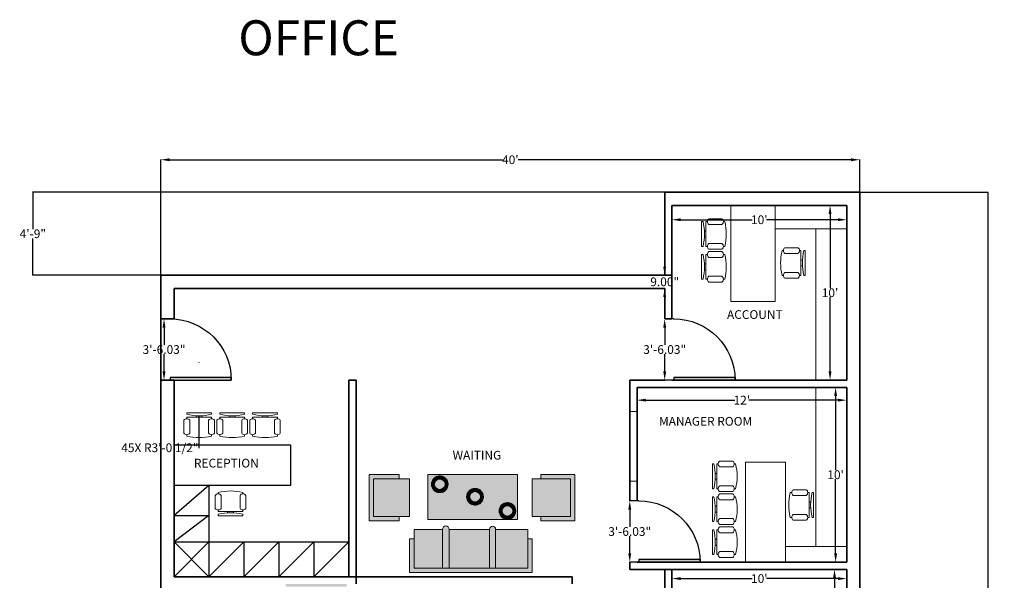
# Model space of a CAD drawing. Units: inches. Extents: x -57 to 1512, y -896 to 149.
# Tile 6 of 6: x 835 to 1512, y -261 to 124. Entities that reach past the tile are written whole.
import ezdxf

# ---------------------------------------------------------------- set-up
doc = ezdxf.new("R2010")
doc.units = ezdxf.units.IN
doc.header["$MEASUREMENT"] = 0
doc.layers.get('Defpoints').update_dxf_attribs({"color": 9})
for name, color, linetype, lineweight in [('A-ANNO-DIMS', 2, 'Continuous', 18), ('A-ANNO-TITL', 7, 'Continuous', 35), ('A-AREA-IDEN', 7, 'Continuous', 18), ('A-DOOR', 3, 'Continuous', 25), ('A-DOOR-PATT', 3, 'Continuous', 13), ('A-FLOR-CASE', 8, 'Continuous', 25), ('A-FURN', 8, 'Continuous', 18), ('A-FURN-PATT', 8, 'Continuous', 13), ('A-GLAZ', 4, 'Continuous', 18), ('A-WALL', 7, 'Continuous', 35)]:
    doc.layers.add(name, color=color, linetype=linetype, lineweight=lineweight)
doc.layers.add('Layer3', color=8, linetype='Continuous')
doc.styles.get("Standard").update_dxf_attribs({"font": 'arial.ttf'})
doc.dimstyles.get("Standard").update_dxf_attribs({"dimtxt": 6, "dimasz": 0.18, "dimexe": 0.18, "dimexo": 0.0625, "dimgap": 0.09, "dimtad": 0, "dimtih": 1, "dimtoh": 1, "dimzin": 0, "dimdsep": 46, "dimlunit": 3, "dimtxsty": 'Standard', "dimcen": 0.09, "dimadec": 0, "dimazin": 0, "dimtfac": 1, "dimtofl": 0, "dimtmove": 0, "dimatfit": 3, "dimfxl": 1, "dimtolj": 1, "dimtzin": 0, "dimarcsym": 0})

# ---------------------------------------------------------------- blocks, each defined once
blk = doc.blocks.new('*U2')
for p, q in [((0, 0), (0, -6)), ((40, 0), (40, -6))]:
    blk.add_line(p, q)
blk.add_lwpolyline([(0, 0), (0, 40), (1.75, 40), (1.75, 0)], close=True)
blk.add_arc((0, 0), 40, 0, 90)
blk = doc.blocks.new('*D35')
at = {"layer": 'A-ANNO-DIMS', "color": 0, "lineweight": -2, "transparency": 16777216}
for p, q in [((1254.53, -206.39), (1254.65, -206.39)), ((1254.47, -212.39), (1254.47, -224.25)), ((1254.47, -242.42), (1254.47, -230.56)), ((1254.53, -248.42), (1254.65, -248.42))]:
    blk.add_line(p, q, dxfattribs=at)
at = {"layer": 'A-ANNO-DIMS', "color": 0, "transparency": 16777216}
for points in [[(1253.47, -212.39), (1255.47, -212.39), (1254.47, -206.39)], [(1253.47, -242.42), (1255.47, -242.42), (1254.47, -248.42)]]:
    blk.add_solid(points, dxfattribs=at)
at = {"layer": 'Defpoints', "color": 0, "transparency": 16777216}
for p in [(1254.47, -206.39), (1254.47, -206.39), (1254.47, -248.42)]:
    blk.add_point(p, dxfattribs=at)
at = {"layer": 'A-ANNO-DIMS', "color": 0, "transparency": 16777216, "insert": (1254.47, -227.41), "char_height": 6, "attachment_point": 5}
blk.add_mtext('\\A1;3\'-6.03"', dxfattribs=at)
blk = doc.blocks.new('*D36')
at = {"layer": 'A-ANNO-DIMS', "color": 0, "lineweight": -2, "transparency": 16777216}
for p, q in [((1278.47, -87.39), (1278.47, -99.25)), ((1278.53, -81.39), (1278.65, -81.39)), ((1278.47, -117.42), (1278.47, -105.56)), ((1278.53, -123.42), (1278.65, -123.42))]:
    blk.add_line(p, q, dxfattribs=at)
at = {"layer": 'A-ANNO-DIMS', "color": 0, "transparency": 16777216}
for points in [[(1277.47, -87.39), (1279.47, -87.39), (1278.47, -81.39)], [(1277.47, -117.42), (1279.47, -117.42), (1278.47, -123.42)]]:
    blk.add_solid(points, dxfattribs=at)
at = {"layer": 'Defpoints', "color": 0, "transparency": 16777216}
for p in [(1278.47, -81.39), (1278.47, -123.42), (1278.47, -123.42)]:
    blk.add_point(p, dxfattribs=at)
at = {"layer": 'A-ANNO-DIMS', "color": 0, "transparency": 16777216, "insert": (1278.47, -102.41), "char_height": 6, "attachment_point": 5}
blk.add_mtext('\\A1;3\'-6.03"', dxfattribs=at)
blk = doc.blocks.new('*D37')
at = {"layer": 'A-ANNO-DIMS', "color": 0, "lineweight": -2, "transparency": 16777216}
for p, q in [((932.53, -81.39), (934.8, -81.39)), ((934.62, -87.39), (934.62, -99.25)), ((934.62, -117.42), (934.62, -105.56)), ((932.53, -123.42), (934.8, -123.42))]:
    blk.add_line(p, q, dxfattribs=at)
at = {"layer": 'A-ANNO-DIMS', "color": 0, "transparency": 16777216}
for points in [[(933.62, -87.39), (935.62, -87.39), (934.62, -81.39)], [(933.62, -117.42), (935.62, -117.42), (934.62, -123.42)]]:
    blk.add_solid(points, dxfattribs=at)
at = {"layer": 'Defpoints', "color": 0, "transparency": 16777216}
for p in [(932.47, -81.39), (932.47, -123.42), (934.62, -123.42)]:
    blk.add_point(p, dxfattribs=at)
at = {"layer": 'A-ANNO-DIMS', "color": 0, "transparency": 16777216, "insert": (934.62, -102.41), "char_height": 6, "attachment_point": 5}
blk.add_mtext('\\A1;3\'-6.03"', dxfattribs=at)
blk = doc.blocks.new('Chair - Desk')
for p, q in [((-8.5, 0), (-8.5, -1)), ((-8.5, 0), (8.5, 0)), ((8.5, 0), (8.5, -1)), ((-10.5, -5), (-10.5, -14)), ((-8.5, -3), (-8.5, -4)), ((-8.5, -3), (8.5, -3)), ((-6.5, -14), (-6.5, -5)), ((-2, -3), (-2, -1.9355)), ((2, -1.9576), (2, -3)), ((6.5, -5), (6.5, -14)), ((8.5, -3), (8.5, -4)), ((10.5, -14), (10.5, -5)), ((-8.5, -15), (-8.5, -16)), ((8.5, -15), (8.5, -16))]:
    blk.add_line(p, q)
for centre, radius, start, end in [((-8.5, -6.5), 2.5, 36.8699, 143.1301), ((0, 34.625), 36.625, 256.5803, 283.4197), ((8.5, -6.5), 2.5, 36.8699, 143.1301), ((-8.5, -12.5), 2.5, 216.8699, 323.1301), ((0, 19.625), 36.625, 256.5803, 283.4197), ((8.5, -12.5), 2.5, 216.8699, 323.1301)]:
    blk.add_arc(centre, radius, start, end)
blk = doc.blocks.new('*U50')
at = {"layer": 'Layer3'}
blk.add_lwpolyline([(0, 4.75, 0.385507), (0, 2.75, 0.385507)], format="xyb", close=True, dxfattribs=at)
blk.add_circle((0, -1), 3.75, dxfattribs=at)
blk = doc.blocks.new('*U51')
at = {"layer": 'A-FURN', "transparency": 16777216}
for p, rotation in [((1143.13, -167.64), 57.6), ((1143.2, -167.54), 50.40000000000002), ((1143.29, -167.44), 43.20000000000001), ((1143.38, -167.36), 36.00000000000001), ((1143.49, -167.3), 28.79999999999998), ((1143.6, -167.24), 21.59999999999999), ((1144.65, -167.44), 316.8), ((1144.74, -167.54), 309.6), ((1144.56, -167.36), 324.0000000000001), ((1144.81, -167.64), 302.4), ((1144.45, -167.3), 331.2), ((1143.72, -167.2), 14.39999999999998), ((1144.34, -167.24), 338.4), ((1144.22, -167.2), 345.6), ((1143.85, -167.18), 7.199999999999979), ((1144.1, -167.18), 352.8), ((1143.13, -168.71), 122.4), ((1143.2, -168.81), 129.6), ((1143.07, -167.75), 64.79999999999998), ((1143.07, -168.6), 115.2), ((1143.29, -168.9), 136.8), ((1143.02, -167.86), 72), ((1143.02, -168.48), 108), ((1143.38, -168.98), 144), ((1142.99, -167.99), 79.2), ((1142.99, -168.36), 100.8), ((1143.49, -169.05), 151.2), ((1142.97, -168.11), 86.40000000000002), ((1142.97, -168.24), 93.60000000000001), ((1143.6, -169.1), 158.4), ((1144.65, -168.9), 223.2), ((1144.74, -168.81), 230.4), ((1144.56, -168.98), 216), ((1144.81, -168.71), 237.6), ((1144.45, -169.05), 208.8), ((1143.72, -169.14), 165.6), ((1144.88, -167.75), 295.2), ((1144.88, -168.6), 244.8), ((1144.34, -169.1), 201.6), ((1144.92, -167.86), 288), ((1144.92, -168.48), 252), ((1144.22, -169.14), 194.4), ((1143.85, -169.16), 172.8000000000001), ((1144.95, -167.99), 280.8), ((1144.95, -168.36), 259.2), ((1144.1, -169.16), 187.1999999999999), ((1144.97, -168.11), 273.6), ((1144.97, -168.24), 266.4000000000001), ((1143.97, -169.17), 180)]:
    blk.add_blockref('*U50', p, dxfattribs=dict(at, rotation=rotation))
blk.add_blockref('*U50', (1143.97, -167.17), dxfattribs=at)
blk = doc.blocks.new('*U52')
at = {"layer": 'Layer3'}
blk.add_lwpolyline([(0, 4.75, 0.385507), (0, 2.75, 0.385507)], format="xyb", close=True, dxfattribs=at)
blk.add_circle((0, -1), 3.75, dxfattribs=at)
blk = doc.blocks.new('*U53')
at = {"layer": 'A-FURN', "transparency": 16777216}
for p, rotation in [((1143.13, -167.64), 57.6), ((1143.2, -167.54), 50.40000000000002), ((1143.29, -167.44), 43.20000000000001), ((1143.38, -167.36), 36.00000000000001), ((1143.49, -167.3), 28.79999999999998), ((1143.6, -167.24), 21.59999999999999), ((1144.65, -167.44), 316.8), ((1144.74, -167.54), 309.6), ((1144.56, -167.36), 324.0000000000001), ((1144.81, -167.64), 302.4), ((1144.45, -167.3), 331.2), ((1143.72, -167.2), 14.39999999999998), ((1144.34, -167.24), 338.4), ((1144.22, -167.2), 345.6), ((1143.85, -167.18), 7.199999999999979), ((1144.1, -167.18), 352.8), ((1143.13, -168.71), 122.4), ((1143.2, -168.81), 129.6), ((1143.07, -167.75), 64.79999999999998), ((1143.07, -168.6), 115.2), ((1143.29, -168.9), 136.8), ((1143.02, -167.86), 72), ((1143.02, -168.48), 108), ((1143.38, -168.98), 144), ((1142.99, -167.99), 79.2), ((1142.99, -168.36), 100.8), ((1143.49, -169.05), 151.2), ((1142.97, -168.11), 86.40000000000002), ((1142.97, -168.24), 93.60000000000001), ((1143.6, -169.1), 158.4), ((1144.65, -168.9), 223.2), ((1144.74, -168.81), 230.4), ((1144.56, -168.98), 216), ((1144.81, -168.71), 237.6), ((1144.45, -169.05), 208.8), ((1143.72, -169.14), 165.6), ((1144.88, -167.75), 295.2), ((1144.88, -168.6), 244.8), ((1144.34, -169.1), 201.6), ((1144.92, -167.86), 288), ((1144.92, -168.48), 252), ((1144.22, -169.14), 194.4), ((1143.85, -169.16), 172.8000000000001), ((1144.95, -167.99), 280.8), ((1144.95, -168.36), 259.2), ((1144.1, -169.16), 187.1999999999999), ((1144.97, -168.11), 273.6), ((1144.97, -168.24), 266.4000000000001), ((1143.97, -169.17), 180)]:
    blk.add_blockref('*U52', p, dxfattribs=dict(at, rotation=rotation))
blk.add_blockref('*U52', (1143.97, -167.17), dxfattribs=at)
blk = doc.blocks.new('*U54')
at = {"layer": 'Layer3'}
blk.add_lwpolyline([(0, 4.75, 0.385507), (0, 2.75, 0.385507)], format="xyb", close=True, dxfattribs=at)
blk.add_circle((0, -1), 3.75, dxfattribs=at)
blk = doc.blocks.new('*U55')
at = {"layer": 'A-FURN', "transparency": 16777216}
for p, rotation in [((1143.13, -167.64), 57.6), ((1143.2, -167.54), 50.40000000000002), ((1143.29, -167.44), 43.20000000000001), ((1143.38, -167.36), 36.00000000000001), ((1143.49, -167.3), 28.79999999999998), ((1143.6, -167.24), 21.59999999999999), ((1144.65, -167.44), 316.8), ((1144.74, -167.54), 309.6), ((1144.56, -167.36), 324.0000000000001), ((1144.81, -167.64), 302.4), ((1144.45, -167.3), 331.2), ((1143.72, -167.2), 14.39999999999998), ((1144.34, -167.24), 338.4), ((1144.22, -167.2), 345.6), ((1143.85, -167.18), 7.199999999999979), ((1144.1, -167.18), 352.8), ((1143.13, -168.71), 122.4), ((1143.2, -168.81), 129.6), ((1143.07, -167.75), 64.79999999999998), ((1143.07, -168.6), 115.2), ((1143.29, -168.9), 136.8), ((1143.02, -167.86), 72), ((1143.02, -168.48), 108), ((1143.38, -168.98), 144), ((1142.99, -167.99), 79.2), ((1142.99, -168.36), 100.8), ((1143.49, -169.05), 151.2), ((1142.97, -168.11), 86.40000000000002), ((1142.97, -168.24), 93.60000000000001), ((1143.6, -169.1), 158.4), ((1144.65, -168.9), 223.2), ((1144.74, -168.81), 230.4), ((1144.56, -168.98), 216), ((1144.81, -168.71), 237.6), ((1144.45, -169.05), 208.8), ((1143.72, -169.14), 165.6), ((1144.88, -167.75), 295.2), ((1144.88, -168.6), 244.8), ((1144.34, -169.1), 201.6), ((1144.92, -167.86), 288), ((1144.92, -168.48), 252), ((1144.22, -169.14), 194.4), ((1143.85, -169.16), 172.8000000000001), ((1144.95, -167.99), 280.8), ((1144.95, -168.36), 259.2), ((1144.1, -169.16), 187.1999999999999), ((1144.97, -168.11), 273.6), ((1144.97, -168.24), 266.4000000000001), ((1143.97, -169.17), 180)]:
    blk.add_blockref('*U54', p, dxfattribs=dict(at, rotation=rotation))
blk.add_blockref('*U54', (1143.97, -167.17), dxfattribs=at)
blk = doc.blocks.new('*D62')
at = {"layer": 'A-ANNO-DIMS', "color": 0, "lineweight": -2, "transparency": 16777216}
for p, q in [((1283.47, -253.48), (1283.47, -259.92)), ((1403.47, -253.48), (1403.47, -259.92)), ((1289.47, -259.74), (1338.57, -259.74)), ((1397.47, -259.74), (1348.37, -259.74))]:
    blk.add_line(p, q, dxfattribs=at)
at = {"layer": 'A-ANNO-DIMS', "color": 0, "transparency": 16777216}
for points in [[(1289.47, -258.74), (1289.47, -260.74), (1283.47, -259.74)], [(1397.47, -258.74), (1397.47, -260.74), (1403.47, -259.74)]]:
    blk.add_solid(points, dxfattribs=at)
at = {"layer": 'Defpoints', "color": 0, "transparency": 16777216}
for p in [(1283.47, -253.42), (1403.47, -253.42), (1403.47, -259.74)]:
    blk.add_point(p, dxfattribs=at)
at = {"layer": 'A-ANNO-DIMS', "color": 0, "transparency": 16777216, "insert": (1343.47, -259.74), "char_height": 6, "attachment_point": 5}
blk.add_mtext("\\A1;10'", dxfattribs=at)
blk = doc.blocks.new('*D63')
at = {"layer": 'A-ANNO-DIMS', "color": 0, "lineweight": -2, "transparency": 16777216}
for p, q in [((1403.41, -253.42), (1394.93, -253.42)), ((1395.11, -259.42), (1395.11, -280.28)), ((1395.11, -307.42), (1395.11, -286.56)), ((1403.41, -313.42), (1394.93, -313.42))]:
    blk.add_line(p, q, dxfattribs=at)
at = {"layer": 'A-ANNO-DIMS', "color": 0, "transparency": 16777216}
for points in [[(1394.11, -259.42), (1396.11, -259.42), (1395.11, -253.42)], [(1394.11, -307.42), (1396.11, -307.42), (1395.11, -313.42)]]:
    blk.add_solid(points, dxfattribs=at)
at = {"layer": 'Defpoints', "color": 0, "transparency": 16777216}
for p in [(1395.11, -253.42), (1403.47, -253.42), (1403.47, -313.42)]:
    blk.add_point(p, dxfattribs=at)
at = {"layer": 'A-ANNO-DIMS', "color": 0, "transparency": 16777216, "insert": (1395.11, -283.42), "char_height": 6, "attachment_point": 5}
blk.add_mtext("\\A1;5'", dxfattribs=at)
blk = doc.blocks.new('*D79')
at = {"layer": 'A-ANNO-DIMS', "color": 0, "lineweight": -2, "transparency": 16777216}
for p, q in [((1259.47, -128.48), (1259.47, -137.37)), ((1403.47, -128.48), (1403.47, -137.37)), ((1265.47, -137.19), (1326.57, -137.19)), ((1397.47, -137.19), (1336.37, -137.19))]:
    blk.add_line(p, q, dxfattribs=at)
at = {"layer": 'A-ANNO-DIMS', "color": 0, "transparency": 16777216}
for points in [[(1265.47, -136.19), (1265.47, -138.19), (1259.47, -137.19)], [(1397.47, -136.19), (1397.47, -138.19), (1403.47, -137.19)]]:
    blk.add_solid(points, dxfattribs=at)
at = {"layer": 'Defpoints', "color": 0, "transparency": 16777216}
for p in [(1259.47, -128.42), (1403.47, -128.42), (1403.47, -137.19)]:
    blk.add_point(p, dxfattribs=at)
at = {"layer": 'A-ANNO-DIMS', "color": 0, "transparency": 16777216, "insert": (1331.47, -137.19), "char_height": 6, "attachment_point": 5}
blk.add_mtext("\\A1;12'", dxfattribs=at)
blk = doc.blocks.new('*D80')
at = {"layer": 'A-ANNO-DIMS', "color": 0, "lineweight": -2, "transparency": 16777216}
for p, q in [((1403.41, -128.42), (1395.7, -128.42)), ((1395.88, -134.42), (1395.88, -185.27)), ((1395.88, -242.42), (1395.88, -191.57)), ((1403.41, -248.42), (1395.7, -248.42))]:
    blk.add_line(p, q, dxfattribs=at)
at = {"layer": 'A-ANNO-DIMS', "color": 0, "transparency": 16777216}
for points in [[(1394.88, -134.42), (1396.88, -134.42), (1395.88, -128.42)], [(1394.88, -242.42), (1396.88, -242.42), (1395.88, -248.42)]]:
    blk.add_solid(points, dxfattribs=at)
at = {"layer": 'Defpoints', "color": 0, "transparency": 16777216}
for p in [(1395.88, -128.42), (1403.47, -128.42), (1403.47, -248.42)]:
    blk.add_point(p, dxfattribs=at)
at = {"layer": 'A-ANNO-DIMS', "color": 0, "transparency": 16777216, "insert": (1395.88, -188.42), "char_height": 6, "attachment_point": 5}
blk.add_mtext("\\A1;10'", dxfattribs=at)
blk = doc.blocks.new('*D81')
at = {"layer": 'A-ANNO-DIMS', "color": 0, "lineweight": -2, "transparency": 16777216}
for p, q in [((1283.47, -3.48), (1283.47, -13.46)), ((1403.47, -3.48), (1403.47, -13.46)), ((1289.47, -13.28), (1338.57, -13.28)), ((1397.47, -13.28), (1348.37, -13.28))]:
    blk.add_line(p, q, dxfattribs=at)
at = {"layer": 'A-ANNO-DIMS', "color": 0, "transparency": 16777216}
for points in [[(1289.47, -12.28), (1289.47, -14.28), (1283.47, -13.28)], [(1397.47, -12.28), (1397.47, -14.28), (1403.47, -13.28)]]:
    blk.add_solid(points, dxfattribs=at)
at = {"layer": 'Defpoints', "color": 0, "transparency": 16777216}
for p in [(1283.47, -3.42), (1403.47, -3.42), (1403.47, -13.28)]:
    blk.add_point(p, dxfattribs=at)
at = {"layer": 'A-ANNO-DIMS', "color": 0, "transparency": 16777216, "insert": (1343.47, -13.28), "char_height": 6, "attachment_point": 5}
blk.add_mtext("\\A1;10'", dxfattribs=at)
blk = doc.blocks.new('*D82')
at = {"layer": 'A-ANNO-DIMS', "color": 0, "lineweight": -2, "transparency": 16777216}
for p, q in [((1403.23, -3.42), (1391.87, -3.42)), ((1392.05, -9.42), (1392.05, -60.27)), ((1392.05, -117.42), (1392.05, -66.57)), ((1403.41, -123.42), (1391.87, -123.42))]:
    blk.add_line(p, q, dxfattribs=at)
at = {"layer": 'A-ANNO-DIMS', "color": 0, "transparency": 16777216}
for points in [[(1391.05, -9.42), (1393.05, -9.42), (1392.05, -3.42)], [(1391.05, -117.42), (1393.05, -117.42), (1392.05, -123.42)]]:
    blk.add_solid(points, dxfattribs=at)
at = {"layer": 'Defpoints', "color": 0, "transparency": 16777216}
for p in [(1392.05, -3.42), (1403.29, -3.42), (1403.47, -123.42)]:
    blk.add_point(p, dxfattribs=at)
at = {"layer": 'A-ANNO-DIMS', "color": 0, "transparency": 16777216, "insert": (1392.05, -63.42), "char_height": 6, "attachment_point": 5}
blk.add_mtext("\\A1;10'", dxfattribs=at)
blk = doc.blocks.new('*D83')
at = {"layer": 'A-ANNO-DIMS', "color": 0, "lineweight": -2, "transparency": 16777216}
for p, q in [((1278.47, -45.42), (1278.47, -39.42)), ((1241, -51.42), (1278.65, -51.42)), ((1241, -60.42), (1278.65, -60.42)), ((1278.47, -66.42), (1278.47, -72.42))]:
    blk.add_line(p, q, dxfattribs=at)
at = {"layer": 'A-ANNO-DIMS', "color": 0, "transparency": 16777216}
for points in [[(1277.47, -45.42), (1279.47, -45.42), (1278.47, -51.42)], [(1277.47, -66.42), (1279.47, -66.42), (1278.47, -60.42)]]:
    blk.add_solid(points, dxfattribs=at)
at = {"layer": 'Defpoints', "color": 0, "transparency": 16777216}
for p in [(1240.94, -51.42), (1240.94, -60.42), (1278.47, -60.42)]:
    blk.add_point(p, dxfattribs=at)
at = {"layer": 'A-ANNO-DIMS', "color": 0, "transparency": 16777216, "insert": (1278.47, -55.92), "char_height": 6, "attachment_point": 5}
blk.add_mtext('\\A1;9.00"', dxfattribs=at)
blk = doc.blocks.new('*D84')
at = {"layer": 'A-ANNO-DIMS', "color": 0, "lineweight": -2, "transparency": 16777216}
for p, q in [((932.47, -51.36), (932.47, 28.11)), ((938.47, 27.93), (1167.17, 27.93)), ((1406.47, 27.93), (1177.77, 27.93)), ((1412.47, -51.36), (1412.47, 28.11))]:
    blk.add_line(p, q, dxfattribs=at)
at = {"layer": 'A-ANNO-DIMS', "color": 0, "transparency": 16777216}
for points in [[(938.47, 28.93), (938.47, 26.93), (932.47, 27.93)], [(1406.47, 28.93), (1406.47, 26.93), (1412.47, 27.93)]]:
    blk.add_solid(points, dxfattribs=at)
at = {"layer": 'Defpoints', "color": 0, "transparency": 16777216}
for p in [(1412.47, 27.93), (932.47, -51.42), (1412.47, -51.42)]:
    blk.add_point(p, dxfattribs=at)
at = {"layer": 'A-ANNO-DIMS', "color": 0, "transparency": 16777216, "insert": (1172.47, 27.93), "char_height": 6, "attachment_point": 5}
blk.add_mtext("\\A1;40'", dxfattribs=at)
blk = doc.blocks.new('*D105')
at = {"layer": 'A-ANNO-DIMS', "color": 0, "lineweight": -2, "transparency": 16777216}
for p, q in [((1412.53, 5.58), (1500.6, 5.58)), ((1500.42, 5.4), (1500.42, -297.27)), ((1500.42, -606.24), (1500.42, -303.57)), ((1412.53, -606.42), (1500.6, -606.42))]:
    blk.add_line(p, q, dxfattribs=at)
at = {"layer": 'A-ANNO-DIMS', "color": 0, "transparency": 16777216}
for points in [[(1500.39, 5.4), (1500.45, 5.4), (1500.42, 5.58)], [(1500.39, -606.24), (1500.45, -606.24), (1500.42, -606.42)]]:
    blk.add_solid(points, dxfattribs=at)
at = {"layer": 'Defpoints', "color": 0, "transparency": 16777216}
for p in [(1412.47, 5.58), (1500.42, 5.58), (1412.47, -606.42)]:
    blk.add_point(p, dxfattribs=at)
at = {"layer": 'A-ANNO-DIMS', "color": 0, "transparency": 16777216, "insert": (1500.42, -300.42), "char_height": 6, "attachment_point": 5}
blk.add_mtext('\\A1;51\'-0"', dxfattribs=at)
blk = doc.blocks.new('*D106')
at = {"layer": 'A-ANNO-DIMS', "color": 0, "lineweight": -2, "transparency": 16777216}
for p, q in [((1278.41, 5.58), (844.34, 5.58)), ((844.52, 5.4), (844.52, -19.77)), ((844.52, -51.24), (844.52, -26.07)), ((932.41, -51.42), (844.34, -51.42))]:
    blk.add_line(p, q, dxfattribs=at)
at = {"layer": 'A-ANNO-DIMS', "color": 0, "transparency": 16777216}
for points in [[(844.49, 5.4), (844.55, 5.4), (844.52, 5.58)], [(844.49, -51.24), (844.55, -51.24), (844.52, -51.42)]]:
    blk.add_solid(points, dxfattribs=at)
at = {"layer": 'Defpoints', "color": 0, "transparency": 16777216}
for p in [(844.52, 5.58), (1278.47, 5.58), (932.47, -51.42)]:
    blk.add_point(p, dxfattribs=at)
at = {"layer": 'A-ANNO-DIMS', "color": 0, "transparency": 16777216, "insert": (844.52, -22.92), "char_height": 6, "attachment_point": 5}
blk.add_mtext('\\A1;4\'-9"', dxfattribs=at)
blk = doc.blocks.new('*D110')
at = {"layer": 'A-ANNO-DIMS', "color": 0, "lineweight": -2, "transparency": 16777216}
for p, q in [((958.67, -111.29), (958.85, -111.29)), ((958.76, -111.38), (958.76, -111.2)), ((958.76, -169.89), (958.76, -148.09)), ((958.58, -169.89), (958.76, -169.89))]:
    blk.add_line(p, q, dxfattribs=at)
at = {"layer": 'A-ANNO-DIMS', "color": 0, "transparency": 16777216}
blk.add_solid([(958.73, -148.09), (958.79, -148.09), (958.76, -147.91)], dxfattribs=at)
at = {"layer": 'Defpoints', "color": 0, "transparency": 16777216}
for p in [(958.76, -111.29), (958.76, -147.91)]:
    blk.add_point(p, dxfattribs=at)
at = {"layer": 'A-ANNO-DIMS', "color": 0, "transparency": 16777216, "insert": (931.76, -169.89), "char_height": 6, "attachment_point": 5}
blk.add_mtext('\\A1;45X R3\'-0 1/2"', dxfattribs=at)

msp = doc.modelspace()

# ---------------------------------------------------------------- hatches: boundary and pattern name
at = {"layer": 'A-DOOR-PATT'}
h = msp.add_hatch(color=256, dxfattribs=at)
h.dxf.hatch_style = 1
h.paths.add_polyline_path([(1084.811, -453.421), (1053.741, -453.421, 0.0109414), (1053.771, -454.781), (1084.811, -454.781)])
h.paths.add_polyline_path([(1091.31, -491.725), (1089.471, -491.725), (1089.471, -533.753), (1091.31, -533.753)])
h.paths.add_polyline_path([(1216.31, -514.725), (1214.471, -514.725), (1214.471, -556.753, 0.0109414), (1216.31, -556.713)])
h.paths.add_polyline_path([(1312.941, -507.109), (1282.971, -507.109), (1282.971, -508.421), (1312.969, -508.421, 0.0109414)])
h.paths.add_polyline_path([(1312.941, -442.147), (1282.971, -442.147), (1282.971, -443.421), (1312.969, -443.421, 0.0106229)])
h.paths.add_polyline_path([(1302.763, -246.583), (1260.775, -246.583), (1260.775, -248.421), (1302.803, -248.421, 0.0109414)])
h.paths.add_polyline_path([(1312.941, -312.109), (1282.971, -312.109), (1282.971, -313.421), (1312.969, -313.421, 0.0109414)])
h.paths.add_polyline_path([(1312.941, -377.109), (1282.971, -377.109), (1282.971, -378.421), (1312.969, -378.421, 0.0109414)])
h.paths.add_polyline_path([(1061.471, -387.473), (1060.289, -387.473), (1060.289, -414.461, 0.0109414), (1061.471, -414.487)])
h.paths.add_polyline_path([(1060.167, -263.421), (1018.139, -263.421, 0.0109414), (1018.179, -265.26), (1060.167, -265.26)])
h.paths.add_polyline_path([(1326.803, -121.583), (1284.775, -121.583), (1284.775, -123.421), (1326.803, -123.421)])
h.paths.add_polyline_path([(980.763, -121.583), (938.775, -121.583), (938.775, -123.421), (980.803, -123.421, 0.0109414)])
h.paths.add_polyline_path([(1177.375, -188.23), (1115.807, -188.23), (1115.807, -219.221), (1177.375, -219.221)])
at = {"layer": 'A-FURN-PATT'}
h = msp.add_hatch(color=256, dxfattribs=at)
h.dxf.hatch_style = 1
h.paths.add_polyline_path([(1106.308, -232.537), (1103.308, -232.537), (1103.308, -255.55), (1187.559, -255.55), (1187.559, -232.537), (1184.559, -232.537), (1184.559, -252.55), (1106.308, -252.55)])
h.paths.add_polyline_path([(1078.534, -191.23), (1096.192, -191.23), (1096.192, -188.23), (1075.534, -188.23), (1075.534, -220.146), (1096.192, -220.146), (1096.192, -217.146), (1078.534, -217.146)])
h.paths.add_polyline_path([(1216.723, -188.23), (1193.523, -188.23), (1193.523, -191.23), (1213.723, -191.23), (1213.723, -217.146), (1193.523, -217.146), (1193.523, -220.146), (1216.723, -220.146)])
h.paths.add_polyline_path([(1184.559, -225.948), (1162.363, -225.948), (1162.363, -252.55), (1184.559, -252.55)])
h.paths.add_polyline_path([(1158.129, -225.948), (1130.506, -225.948), (1130.506, -252.55), (1158.129, -252.55)])
h.paths.add_polyline_path([(1125.823, -225.948), (1106.308, -225.948), (1106.308, -252.55), (1125.823, -252.55)])
h.paths.add_polyline_path([(1103.308, -191.23), (1078.534, -191.23), (1078.534, -217.146), (1103.308, -217.146)])
h.paths.add_polyline_path([(1213.723, -191.23), (1187.559, -191.23), (1187.559, -217.146), (1213.723, -217.146)])
h = msp.add_hatch(color=256, dxfattribs=at)
h.dxf.hatch_style = 1
h.paths.add_polyline_path([(1078.534, -191.23), (1096.192, -191.23), (1096.192, -188.23), (1075.534, -188.23), (1075.534, -220.146), (1096.192, -220.146), (1096.192, -217.146), (1078.534, -217.146)])
h.paths.add_polyline_path([(1216.723, -188.23), (1193.523, -188.23), (1193.523, -191.23), (1213.723, -191.23), (1213.723, -217.146), (1193.523, -217.146), (1193.523, -220.146), (1216.723, -220.146)])
h.paths.add_polyline_path([(1187.559, -232.537), (1184.559, -232.537), (1184.559, -252.55), (1106.308, -252.55), (1106.308, -232.537), (1103.308, -232.537), (1103.308, -255.55), (1187.559, -255.55)])
h.paths.add_polyline_path([(1162.363, -225.948, 1), (1158.129, -225.948), (1158.129, -252.55), (1162.363, -252.55)])
h.paths.add_polyline_path([(1130.506, -225.948, 1), (1125.823, -225.948), (1125.823, -252.55), (1130.506, -252.55)])

# ---------------------------------------------------------------- linework, layer by layer
at = {"layer": 'A-FLOR-CASE'}
for p, q in [((941.471, -195.801), (941.471, -258.421)), ((965.471, -195.801), (941.471, -216.421)), ((965.471, -195.801), (965.471, -258.421)), ((941.471, -216.421), (965.471, -216.421)), ((965.471, -216.421), (941.471, -234.421)), ((941.471, -234.421), (1061.471, -234.421)), ((965.471, -234.421), (941.471, -258.421)), ((941.471, -234.421), (965.471, -258.421)), ((989.471, -234.421), (965.471, -258.421)), ((989.471, -234.421), (989.471, -258.421)), ((1013.471, -234.421), (989.471, -258.421)), ((1013.471, -234.421), (1013.471, -258.421)), ((1037.471, -234.421), (1013.471, -258.421)), ((1037.471, -234.421), (1037.471, -258.421)), ((1061.471, -234.421), (1037.471, -258.421))]:
    msp.add_line(p, q, dxfattribs=at)
msp.add_lwpolyline([(941.471, -167.893), (1021.416, -167.893), (1021.416, -195.801), (941.471, -195.801)], close=True, dxfattribs=at)
at = {"layer": 'A-FURN'}
for p, q in [((1096.192, -188.23), (1096.192, -191.23)), ((1193.523, -188.23), (1193.523, -191.23)), ((1096.192, -217.146), (1096.192, -220.146)), ((1193.523, -217.146), (1193.523, -220.146)), ((1125.823, -225.948), (1125.823, -252.55)), ((1130.506, -225.948), (1130.506, -252.55)), ((1158.129, -252.55), (1158.129, -225.948)), ((1162.363, -252.55), (1162.363, -225.948)), ((1103.308, -232.537), (1106.308, -232.537)), ((1184.559, -232.537), (1187.559, -232.537)), ((1125.823, -252.55), (1162.363, -252.55)), ((1130.506, -252.55), (1158.129, -252.55))]:
    msp.add_line(p, q, dxfattribs=at)
for points in [[(1354.44, -3.421), (1323.851, -3.421), (1323.851, -69.429), (1354.44, -69.429)], [(1403.471, -3.421), (1354.44, -3.421), (1354.44, -19.559), (1403.471, -19.559)], [(1403.471, -19.559), (1382.269, -19.559), (1382.269, -123.421), (1403.471, -123.421)], [(1382.269, -128.421), (1403.471, -128.421), (1403.471, -237.749), (1382.269, -237.749)], [(1361.436, -248.421), (1334.047, -248.421), (1334.047, -179.751), (1361.436, -179.751)], [(1115.807, -188.23), (1177.375, -188.23), (1177.375, -219.221), (1115.807, -219.221)], [(1403.471, -237.749), (1361.436, -237.749), (1361.436, -248.421), (1403.471, -248.421)], [(1403.471, -237.749), (1403.471, -237.749), (1403.471, -248.421), (1403.471, -248.421)]]:
    msp.add_lwpolyline(points, close=True, dxfattribs=at)
for points in [[(1096.192, -188.23), (1075.534, -188.23), (1075.534, -220.146), (1096.192, -220.146)], [(1193.523, -188.23), (1216.723, -188.23), (1216.723, -220.146), (1193.523, -220.146)], [(1103.308, -191.23), (1078.534, -191.23), (1078.534, -217.146), (1103.308, -217.146)], [(1103.308, -217.146), (1103.308, -191.23)], [(1187.559, -191.23), (1213.723, -191.23), (1213.723, -217.146), (1187.559, -217.146)], [(1187.559, -217.146), (1187.559, -191.23)], [(1106.308, -225.948), (1125.823, -225.948)], [(1184.559, -225.948), (1184.559, -252.55), (1106.308, -252.55), (1106.308, -225.948)], [(1130.506, -225.948), (1158.129, -225.948)], [(1162.363, -225.948), (1184.559, -225.948)], [(1187.559, -232.537), (1187.559, -255.55), (1103.308, -255.55), (1103.308, -232.537)]]:
    msp.add_lwpolyline(points, dxfattribs=at)
for centre in [(1123.971, -194.973), (1148.221, -203.516), (1170.45, -213.302)]:
    msp.add_circle(centre, 5.75, dxfattribs=at)
for centre, radius in [((1128.165, -225.948), 2.342), ((1160.246, -225.948), 2.117)]:
    msp.add_arc(centre, radius, 0, 180, dxfattribs=at)
at = {"layer": 'A-GLAZ'}
for p, q in [((1254.442, -144.907), (1259.471, -144.907)), ((1254.442, -192.907), (1259.471, -192.907))]:
    msp.add_line(p, q, dxfattribs=at)
at = {"layer": 'A-WALL'}
for p, q in [((1278.471, 5.579), (1412.471, 5.579)), ((1278.471, 5.579), (1278.471, -51.421)), ((1412.471, 5.579), (1412.471, -318.421)), ((1283.471, -3.421), (1403.471, -3.421)), ((1283.471, -3.421), (1283.471, -81.421)), ((1403.471, -3.421), (1403.471, -123.421)), ((932.471, -51.421), (932.471, -606.421)), ((932.471, -51.421), (1278.471, -51.421)), ((1278.471, -51.421), (1283.471, -51.421)), ((941.471, -60.421), (941.471, -81.48)), ((941.471, -60.421), (1278.471, -60.421)), ((1278.471, -60.421), (1278.471, -81.421)), ((932.471, -81.421), (941.471, -81.421)), ((1278.471, -81.421), (1283.471, -81.421)), ((932.471, -123.421), (941.471, -123.421)), ((941.471, -123.421), (941.471, -258.421)), ((1061.471, -123.421), (1061.471, -258.421)), ((1061.471, -123.421), (1066.471, -123.421)), ((1066.471, -123.421), (1066.471, -263.421)), ((1254.471, -123.421), (1254.471, -206.393)), ((1254.471, -123.421), (1278.471, -123.421)), ((1259.471, -128.421), (1403.471, -128.421)), ((1259.471, -128.421), (1259.471, -206.393)), ((1283.471, -123.421), (1403.471, -123.421)), ((1403.471, -128.421), (1403.471, -248.421)), ((1254.471, -248.421), (1254.471, -253.421)), ((1259.471, -248.421), (1403.471, -248.421)), ((1254.471, -253.421), (1403.471, -253.421)), ((1278.471, -253.421), (1278.471, -348.423)), ((1283.471, -253.421), (1283.471, -283.607)), ((1403.471, -253.421), (1403.471, -313.421)), ((941.471, -258.421), (1214.89, -258.421)), ((1214.89, -258.421), (1214.89, -263.421))]:
    msp.add_line(p, q, dxfattribs=at)

# ---------------------------------------------------------------- block references
at = {"layer": 'A-DOOR', "xscale": -1.050697738247698, "yscale": 1.050697738247698, "zscale": 1.050697738247698, "rotation": 270}
for p in [(938.775, -123.421), (1284.775, -123.421), (1260.775, -248.421)]:
    msp.add_blockref('*U2', p, dxfattribs=at)
at = {"layer": 'A-FURN'}
for p, rotation in [((1303.801, -23.053), 90), ((1303.801, -45.636), 90), ((1311.22, -189.52), 90), ((980.315, -216.568), 180), ((1311.22, -212.04), 90), ((1311.22, -234.739), 90)]:
    msp.add_blockref('Chair - Desk', p, dxfattribs=dict(at, rotation=rotation))
at = {"layer": 'A-FURN', "xscale": -1, "rotation": 270}
for p in [(1375.071, -42.971), (1380.736, -209.184)]:
    msp.add_blockref('Chair - Desk', p, dxfattribs=at)
at = {"layer": 'A-FURN'}
for name, p in [('Chair - Desk', (958.764, -145.913)), ('Chair - Desk', (981.463, -145.913)), ('Chair - Desk', (1003.983, -145.913)), ('*U51', (-19.999, -26.801)), ('*U55', (4.251, -35.344)), ('*U53', (26.48, -45.13))]:
    msp.add_blockref(name, p, dxfattribs=at)

# ---------------------------------------------------------------- texts
at = {"layer": 'A-ANNO-TITL', "insert": (985.642, 123.689), "char_height": 24, "attachment_point": 1}
msp.add_mtext_dynamic_manual_height_columns('OFFICE', width=777.91361, gutter_width=1, heights=[0], dxfattribs=at)
at = {"layer": 'A-AREA-IDEN', "char_height": 6, "attachment_point": 1}
for s, insert in [('ACCOUNT', (1321.272, -75.398)), ('MANAGER ROOM', (1274.59, -148.713)), ('WAITING', (1132.818, -171.992)), ('RECEPTION', (955.136, -177.45))]:
    msp.add_mtext_dynamic_manual_height_columns(s, width=160.11736, gutter_width=1, heights=[0], dxfattribs=dict(at, insert=insert))

# ---------------------------------------------------------------- dimensions: what is measured, and where the dimension line sits
at = {"layer": 'A-ANNO-DIMS'}
for base, p1, p2, picture, middle in [((1412.471, 27.934), (932.471, -51.421), (1412.471, -51.421), '*D84', (1172.471, 27.934)), ((1403.471, -13.278), (1283.471, -3.421), (1403.471, -3.421), '*D81', (1343.471, -13.278)), ((1403.471, -137.191), (1259.471, -128.421), (1403.471, -128.421), '*D79', (1331.471, -137.191)), ((1403.471, -259.741), (1283.471, -253.421), (1403.471, -253.421), '*D62', (1343.471, -259.741))]:
    dim = msp.add_linear_dim(base=base, p1=p1, p2=p2, dimstyle='Standard', override={"dimasz": 6, "dimclrd": 0, "dimclre": 0, "dimclrt": 0}, dxfattribs=at)
    dim.commit()
    dim.dimension.update_dxf_attribs({"geometry": picture, "text_midpoint": middle})
for base, p1, p2, override, picture, middle in [((844.521, 5.579), (932.471, -51.421), (1278.471, 5.579), {"dimdec": 1, "dimlfac": 1, "dimrnd": 0, "dimzin": 1, "dimdsep": 46, "dimlunit": 4, "dimfrac": 2}, '*D106', (844.521, -22.921)), ((1500.421, 5.579), (1412.471, -606.421), (1412.471, 5.579), {"dimdec": 1, "dimlfac": 1, "dimrnd": 0, "dimzin": 1, "dimdsep": 46, "dimlunit": 4, "dimfrac": 2}, '*D105', (1500.421, -300.421)), ((1392.047, -3.421), (1403.471, -123.421), (1403.291, -3.421), {"dimasz": 6, "dimclrd": 0, "dimclre": 0, "dimclrt": 0}, '*D82', (1392.047, -63.421)), ((1278.471, -60.421), (1240.937, -51.421), (1240.937, -60.421), {"dimasz": 6, "dimclrd": 0, "dimclre": 0, "dimclrt": 0}, '*D83', (1278.471, -55.921)), ((934.618, -123.421), (932.471, -81.393), (932.471, -123.421), {"dimasz": 6, "dimclrd": 0, "dimclre": 0, "dimclrt": 0}, '*D37', (934.618, -102.407)), ((1278.471, -123.421), (1278.471, -81.393), (1278.471, -123.421), {"dimasz": 6, "dimclrd": 0, "dimclre": 0, "dimclrt": 0}, '*D36', (1278.471, -102.407)), ((1395.884, -128.421), (1403.471, -248.421), (1403.471, -128.421), {"dimasz": 6, "dimclrd": 0, "dimclre": 0, "dimclrt": 0}, '*D80', (1395.884, -188.421)), ((1254.472, -206.393), (1254.471, -248.421), (1254.471, -206.393), {"dimasz": 6, "dimclrd": 0, "dimclre": 0, "dimclrt": 0}, '*D35', (1254.472, -227.407)), ((1395.11, -253.421), (1403.471, -313.421), (1403.471, -253.421), {"dimasz": 6, "dimclrd": 0, "dimclre": 0, "dimclrt": 0}, '*D63', (1395.11, -283.421))]:
    dim = msp.add_linear_dim(base=base, p1=p1, p2=p2, angle=90, dimstyle='Standard', override=override, dxfattribs=at)
    dim.commit()
    dim.dimension.update_dxf_attribs({"geometry": picture, "text_midpoint": middle})
dim = msp.add_radius_dim(center=(958.764, -111.288), mpoint=(958.764, -147.913), text='45X <>', dimstyle='Standard', override={"dimdec": 1, "dimlfac": 1, "dimrnd": 0, "dimzin": 1, "dimdsep": 46, "dimlunit": 4, "dimfrac": 2}, dxfattribs=at)
dim.commit()
dim.dimension.update_dxf_attribs({"geometry": '*D110', "text_midpoint": (931.76, -169.888), "dimtype": 164})

doc.saveas('drawing.dxf')
